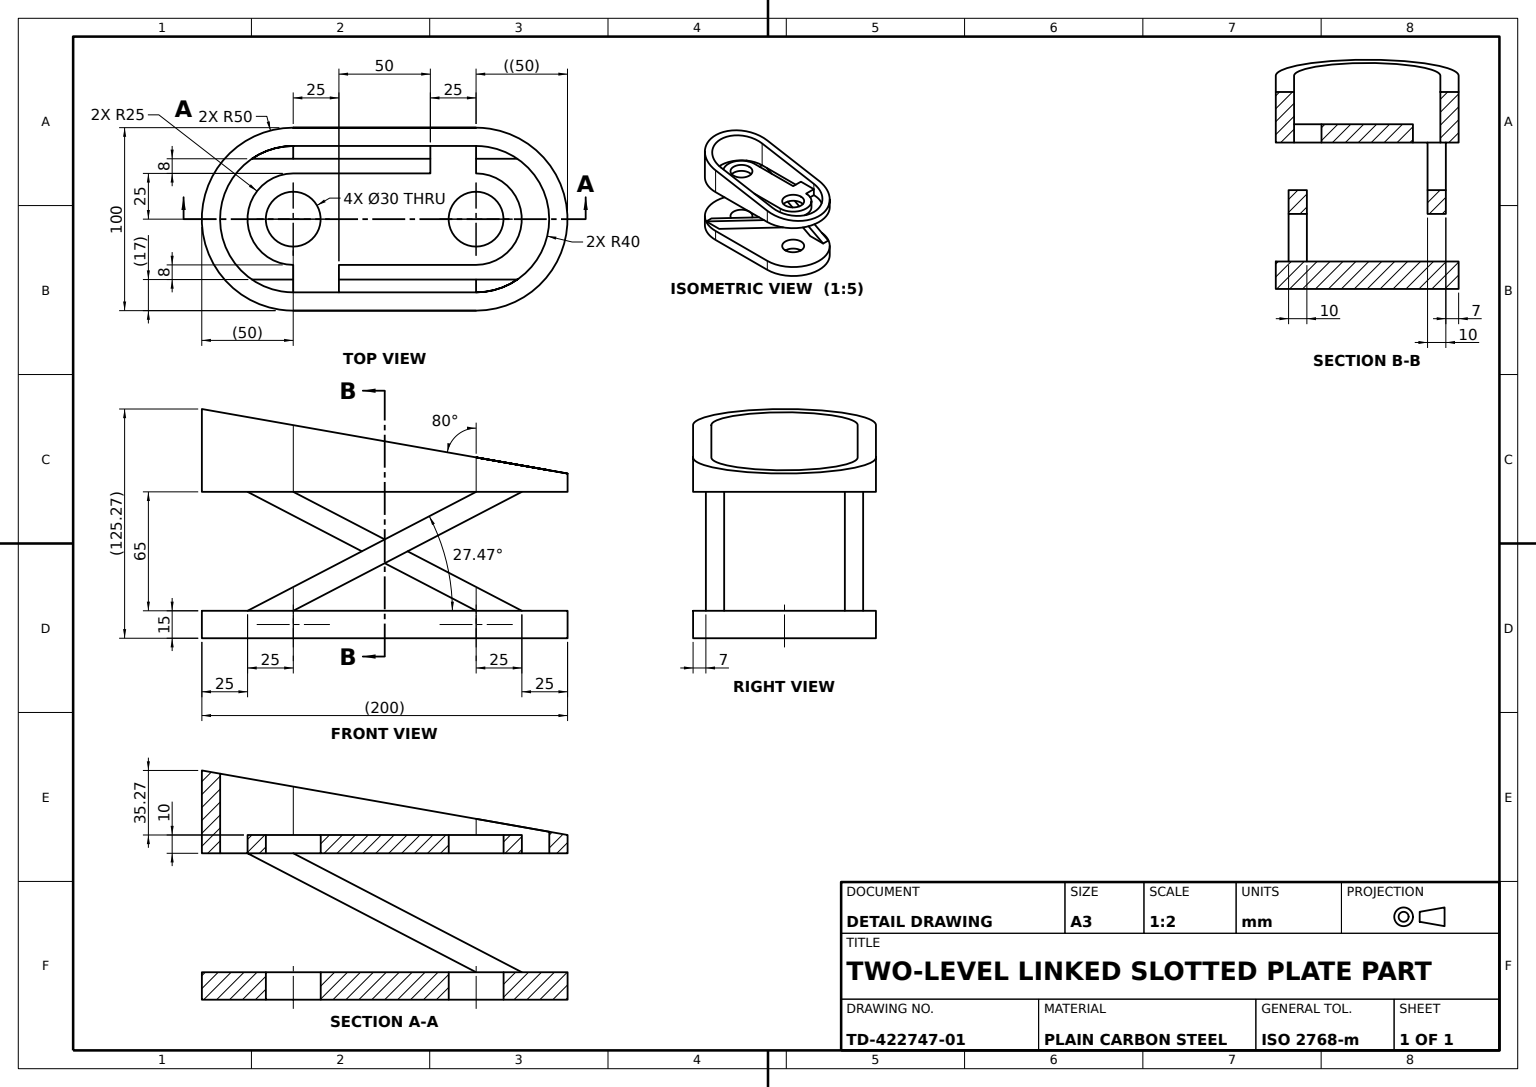
SolidWorks part; units mm, degrees
material "Plain Carbon Steel"
ref_plane "Front Plane" through (0, 0, 0) normal (0, 0, 1) x (1, 0, 0)
ref_plane "Top Plane" through (0, 0, 0) normal (0, 1, 0) x (1, 0, 0)
ref_plane "Right Plane" through (0, 0, 0) normal (1, 0, 0) x (0, 0, -1)
sketch "Base Plate Sketch" plane through (0, 0, 0) normal (0, 1, 0) x (1, 0, 0)
  line L2 (-50, 50) -> (50, 50)
  line L3 (-50, -50) -> (50, -50)
  arc A0 (50, -50) -> (50, 50) centre (50, 0) ccw
  arc A1 (-50, 50) -> (-50, -50) centre (-50, 0) ccw
  dimension "D1" = 50
  dimension "D2" = 100
extrude "Base Plate" add sketch "Base Plate Sketch" along normal blind 15
ref_plane "Upper Plate Plane" through (0, 80, 0) normal (0, 1, 0) x (1, 0, 0)
sketch "Upper Plate Sketch" plane through (0, 80, 0) normal (0, 1, 0) x (1, 0, 0)
  line L0 (50, 50) -> (25, 50)
  line L1 (25, 50) -> (25, 25)
  line L2 (-50, 25) -> (25, 25)
  line L3 (50, 25) -> (50, 50)
  line L4 (-50, -25) -> (50, -25)
  arc A0 (-50, 25) -> (-50, -25) centre (-50, 0) ccw
  arc A1 (50, -25) -> (50, 25) centre (50, 0) ccw
  dimension "D1" = 25
  dimension "D2" = 100
extrude "Upper Plate" add sketch "Upper Plate Sketch" along normal blind 10 separate body
sketch "Loop Wall Sketch" plane through (0, 90, 0) normal (0, 1, 0) x (1, 0, 0)
  line L0 (-50, 50) -> (50, 50)
  line L1 (-50, -50) -> (50, -50)
  line L2 (-50, 40) -> (50, 40)
  line L3 (-50, -40) -> (50, -40)
  arc A0 (-50, 50) -> (-50, -50) centre (-50, 0) ccw
  arc A1 (50, -50) -> (50, 50) centre (50, 0) ccw
  arc A2 (-50, 40) -> (-50, -40) centre (-50, 0) ccw
  arc A3 (50, -40) -> (50, 40) centre (50, 0) ccw
  dimension "D1" = 40
extrude "Loop Wall" add sketch "Loop Wall Sketch" along normal blind 50 and the other way blind 10
sketch "Wall Opening Cut Sketch" plane through (0, 0, 50) normal (0, 0, 1) x (1, 0, 0)
  line L1 (-50, 140) -> (50, 140) construction
  line L2 (100, 90) -> (-100, 125.2654)
  line L3 (-100, 140) -> (-100, 80) construction
  line L4 (-100, 125.2654) -> (-100, 140)
  line L5 (-100, 140) -> (100, 140)
  line L6 (100, 140) -> (100, 90)
  dimension "D1" = 14.7346
  dimension "D2" = 50
extrude "Wall Opening Cut" cut sketch "Wall Opening Cut Sketch" against normal mid plane 320
sketch "Tab Sketch" plane through (0, 0, 25) normal (0, 0, 1) x (1, 0, 0)
  line L0 (-50, 80) -> (-50, 90)
  line L1 (-50, 90) -> (-25, 90)
  line L2 (-25, 90) -> (-25, 80)
  line L3 (-50, 80) -> (50, 80) construction
  line L4 (-25, 80) -> (-50, 80)
  line L5 (50, 90) -> (50, 80) construction
  line L6 (-50, 80) -> (50, 80) construction
  dimension "D1" = 75
  dimension "D2" = 10
extrude "Tab" add sketch "Tab Sketch" along normal blind 20
sketch "Guide Rail 1 Sketch" plane through (0, 0, -40) normal (0, 0, 1) x (1, 0, 0)
  line L0 (50, 15) -> (75, 15)
  line L1 (-50, 15) -> (50, 15) construction
  line L2 (0, 15) -> (75, 15)
  line L3 (100, 15) -> (50, 15) construction
  line L4 (-50, 80) -> (-50, 116.449) construction
  line L9 (-50, 80) -> (-75, 80)
  line L10 (-100, 80) -> (-50, 80) construction
  line L11 (-75, 80) -> (50, 15)
  line L12 (-50, 80) -> (75, 15)
  dimension "D1" = 125
extrude "Guide Rail 1" add sketch "Guide Rail 1 Sketch" along normal blind 7 and the other way blind 3 contours L0 L11 L9 L12
sketch "Guide Rail 2 Sketch" plane through (0, 0, 40) normal (0, 0, -1) x (-1, 0, 0)
  line L1 (50, 90) -> (25, 90) construction
  line L3 (50, 15) -> (75, 15)
  line L4 (100, 15) -> (50, 15) construction
  line L8 (-50, 80) -> (-50, 74.8271)
  line L9 (-50, 80) -> (-75, 80)
  line L10 (-100, 80) -> (-50, 80) construction
  line L11 (-75, 80) -> (50, 15)
  line L12 (-50, 80) -> (75, 15)
  dimension "D1" = 15.1729
extrude "Guide Rail 2" add sketch "Guide Rail 2 Sketch" along normal blind 7 and the other way blind 3 contours L12 L3 L11 L9
sketch "Angled Trim Cut Sketch" plane through (0, 15, 0) normal (0, 1, 0) x (1, 0, 0)
  circle A0 centre (-50, 0) radius 15
  circle A1 centre (50, 0) radius 15
  dimension "D1" = 30
extrude "Angled Trim Cut" cut sketch "Angled Trim Cut Sketch" against normal mid plane 267
